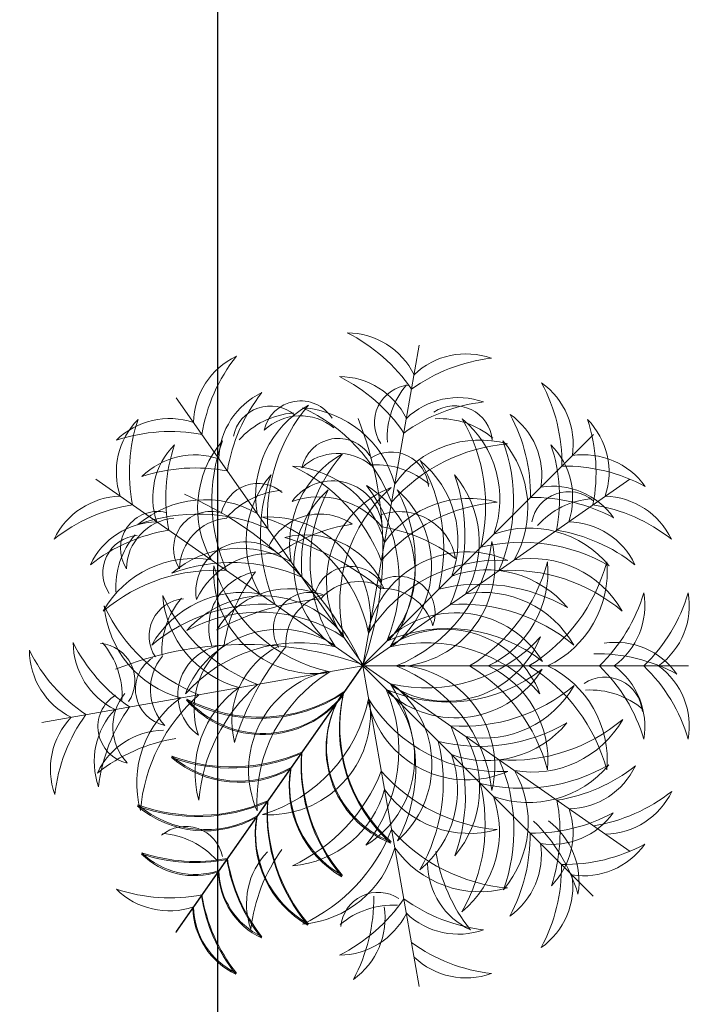
# Model space of a CAD drawing. Units: inches. Extents: x -48 to 50072, y 0 to 21068.
# Tile 18 of 75: x 289 to 316, y 309 to 347. Entities that reach past the tile are written whole.
import ezdxf

# ---------------------------------------------------------------- set-up
doc = ezdxf.new("R2010")
doc.units = ezdxf.units.IN
doc.header["$MEASUREMENT"] = 0
doc.layers.add('A-ANNO-DIMS', color=2, linetype='Continuous', lineweight=18)
doc.layers.add('L-PLNT', color=94, linetype='Continuous', lineweight=13)
doc.styles.get("Standard").update_dxf_attribs({"font": 'arial.ttf'})
doc.dimstyles.get("Standard").update_dxf_attribs({"dimtxt": 8, "dimasz": 0.18, "dimexe": 0.18, "dimexo": 0.0625, "dimgap": 0.09, "dimtad": 0, "dimtih": 1, "dimtoh": 1, "dimdec": 1, "dimzin": 0, "dimdsep": 46, "dimlunit": 4, "dimtxsty": 'Standard', "dimblk": 'ARCHTICK', "dimcen": 0.09, "dimadec": 0, "dimazin": 0, "dimtfac": 1, "dimtdec": 1, "dimtofl": 0, "dimtmove": 0, "dimatfit": 3, "dimldrblk": 'ARCHTICK', "dimfxl": 1, "dimtolj": 1, "dimtzin": 0, "dimarcsym": 0})

# ---------------------------------------------------------------- blocks, each defined once
blk = doc.blocks.new('A$C5D061C3B')
for p, q in [((3.3772, 6.6792), (3.3772, 3.3772)), ((1.4832, 6.082), (3.3772, 3.3772)), ((5.2591, 6.0863), (3.3651, 3.3814)), ((1.0302, 5.7163), (3.3651, 3.3814)), ((5.712, 5.712), (3.3772, 3.3772)), ((0.1253, 3.9506), (3.3772, 3.3772)), ((6.629, 3.9506), (3.3772, 3.3772)), ((0.6603, 1.4875), (3.3651, 3.3814)), ((1.4832, 0.6723), (3.3772, 3.3772)), ((6.0699, 1.4875), (3.3651, 3.3814)), ((3.9506, 0.1253), (3.3772, 3.3772)), ((6.082, 1.4832), (3.3772, 3.3772))]:
    blk.add_line(p, q)
for centre, radius, start, end in [((2.7629, 5.9242), 0.7621, 36.28997, 99.62433), ((2.1448, 5.0319), 1.7154, 44.07628, 73.37936), ((3.9915, 5.9242), 0.7621, 80.37567, 143.71003), ((4.6096, 5.0319), 1.7154, 106.62064, 135.92372), ((2.4194, 5.816), 0.7621, 115.37567, 178.71003), ((3.4376, 5.4395), 1.7154, 141.62064, 170.92372), ((3.9007, 5.9388), 0.7621, 125.37567, 188.71003), ((4.9688, 5.7448), 1.7154, 151.62064, 180.92372), ((3.3047, 5.4438), 1.7154, 9.07628, 38.37936), ((4.3228, 5.8202), 0.7621, 1.28997, 64.62433), ((1.9984, 5.6169), 0.7621, 125.37567, 188.71003), ((3.0665, 5.4229), 1.7154, 151.62064, 180.92372), ((2.7629, 5.4738), 0.7621, 36.28997, 99.62433), ((2.1448, 4.5814), 1.7154, 44.07628, 73.37936), ((3.9915, 5.4738), 0.7621, 80.37567, 143.71003), ((4.6096, 4.5814), 1.7154, 106.62064, 135.92372), ((3.8712, 5.8319), 0.3799, 94.742, 213.74753), ((4.4474, 5.6807), 0.826, 139.61802, 183.21064), ((4.7438, 5.6126), 0.7621, 351.28997, 54.62433), ((3.6758, 5.4187), 1.7154, 359.07628, 28.37936), ((2.6778, 5.4469), 0.7621, 115.37567, 178.71003), ((3.696, 5.0705), 1.7154, 141.62064, 170.92372), ((4.0645, 5.4512), 0.7621, 1.28997, 64.62433), ((3.0463, 5.0747), 1.7154, 9.07628, 38.37936), ((3.3438, 5.0894), 1.0556, 119.60629, 189.75109), ((4.1771, 4.8688), 1.7695, 139.96343, 183.62881), ((3.3985, 5.0936), 1.0556, 350.24891, 60.39371), ((2.5652, 4.8731), 1.7695, 356.37119, 40.03657), ((2.317, 5.2983), 0.7621, 125.37567, 188.71003), ((3.385, 5.1044), 1.7154, 151.62064, 180.92372), ((3.3573, 5.1001), 1.7154, 359.07628, 28.37936), ((4.4253, 5.2941), 0.7621, 351.28997, 54.62433), ((1.413, 5.1113), 0.7621, 71.28997, 134.62433), ((3.0349, 5.0618), 1.0556, 129.60629, 199.75109), ((3.8939, 4.9893), 1.7695, 149.96343, 193.62881), ((2.4224, 4.7989), 1.0556, 25.24891, 95.39371), ((1.8663, 4.1402), 1.7695, 31.37119, 75.03657), ((4.3319, 4.7989), 1.0556, 84.60629, 154.75109), ((4.888, 4.1402), 1.7695, 104.96343, 148.62881), ((2.8484, 4.9851), 1.7695, 346.37119, 30.03657), ((3.7074, 5.0576), 1.0556, 340.24891, 50.39371), ((1.4185, 4.0258), 1.7154, 79.07628, 108.37936), ((1.9907, 5.4623), 0.3799, 139.742, 258.74753), ((2.5051, 5.7628), 0.826, 184.61802, 228.21064), ((1.1297, 4.7481), 0.7621, 81.28997, 144.62433), ((1.6714, 4.7422), 0.7621, 71.28997, 134.62433), ((3.6883, 4.5973), 1.0556, 119.60629, 189.75109), ((4.5216, 4.3768), 1.7695, 139.96343, 183.62881), ((2.2207, 4.3811), 1.7695, 356.37119, 40.03657), ((3.054, 4.6016), 1.0556, 350.24891, 60.39371), ((5.0709, 4.7465), 0.7621, 45.37567, 108.71003), ((5.5642, 4.8068), 0.7621, 80.37567, 143.71003), ((6.1823, 3.9144), 1.7154, 106.62064, 135.92372), ((5.6126, 4.7438), 0.7621, 35.37567, 98.71003), ((1.3236, 3.68), 1.7154, 89.07628, 118.37936), ((3.4596, 4.6371), 1.0556, 129.60629, 199.75109), ((4.3186, 4.5646), 1.7695, 149.96343, 193.62881), ((3.2827, 4.6328), 1.0556, 340.24891, 50.39371), ((2.4237, 4.5604), 1.7695, 346.37119, 30.03657), ((5.4187, 3.6758), 1.7154, 61.62064, 90.92372), ((1.6769, 3.6567), 1.7154, 79.07628, 108.37936), ((5.0653, 3.661), 1.7154, 71.62064, 100.92372), ((1.4482, 4.4296), 0.7621, 81.28997, 144.62433), ((2.4224, 4.1982), 1.0556, 25.24891, 95.39371), ((1.8663, 3.5396), 1.7695, 31.37119, 75.03657), ((3.8676, 4.3207), 1.029, 121.36542, 221.57406), ((4.5556, 4.2369), 1.5567, 141.81221, 203.33354), ((4.3319, 4.1982), 1.0556, 84.60629, 154.75109), ((4.888, 3.5396), 1.7695, 104.96343, 148.62881), ((2.1867, 4.2327), 1.5567, 336.66646, 38.18779), ((2.8746, 4.3165), 1.029, 318.42594, 58.63458), ((4.0352, 4.215), 1.029, 111.36542, 211.57406), ((2.7071, 4.2192), 1.029, 328.42594, 68.63458), ((2.0441, 4.0172), 1.5567, 346.66646, 48.18779), ((4.6982, 4.0129), 1.5567, 131.81221, 193.33354), ((5.2941, 4.4253), 0.7621, 35.37567, 98.71003), ((1.6421, 3.3615), 1.7154, 89.07628, 118.37936), ((1.7796, 3.9941), 1.0556, 60.24891, 130.39371), ((4.9626, 3.9984), 1.0556, 49.60629, 119.75109), ((5.1001, 3.3573), 1.7154, 61.62064, 90.92372), ((1.7019, 3.1357), 1.7695, 66.37119, 110.03657), ((5.0404, 3.1399), 1.7695, 69.96343, 113.62881), ((2.1429, 4.5643), 1.0556, 164.60629, 234.75109), ((2.888, 4.9976), 1.7695, 184.96343, 228.62881), ((3.25, 4.4348), 1.029, 156.36542, 256.57406), ((3.8617, 4.7608), 1.5567, 176.81221, 238.33354), ((2.8927, 4.7608), 1.5567, 301.66646, 3.18779), ((3.5043, 4.4348), 1.029, 283.42594, 23.63458), ((3.8663, 4.9976), 1.7695, 311.37119, 355.03657), ((4.6115, 4.5643), 1.0556, 305.24891, 15.39371), ((1.6965, 4.1589), 0.826, 139.61802, 183.21064), ((1.6847, 3.7116), 1.0556, 70.24891, 140.39371), ((2.7344, 4.46), 1.0556, 164.60629, 234.75109), ((3.4796, 4.8933), 1.7695, 184.96343, 228.62881), ((2.3576, 3.686), 1.029, 3.42594, 103.63458), ((4.3967, 3.686), 1.029, 76.36542, 176.57406), ((3.2748, 4.8933), 1.7695, 311.37119, 355.03657), ((4.02, 4.46), 1.0556, 305.24891, 15.39371), ((5.0576, 3.7074), 1.0556, 39.60629, 109.75109), ((0.9755, 4.4244), 0.7621, 160.37567, 223.71003), ((1.9616, 4.8782), 1.7154, 186.62064, 215.92372), ((1.4191, 4.3462), 0.7621, 160.37567, 223.71003), ((2.4052, 4.8), 1.7154, 186.62064, 215.92372), ((1.1202, 4.3101), 0.3799, 94.742, 213.74753), ((1.7572, 2.8527), 1.7695, 76.37119, 120.03657), ((1.9304, 3.1403), 1.5567, 21.66646, 83.18779), ((4.8239, 3.1403), 1.5567, 96.81221, 158.33354), ((4.9851, 2.8484), 1.7695, 59.96343, 103.62881), ((4.3491, 4.8), 1.7154, 324.07628, 353.37936), ((5.3352, 4.3462), 0.7621, 316.28997, 19.62433), ((4.7927, 4.8782), 1.7154, 324.07628, 353.37936), ((5.7789, 4.4244), 0.7621, 316.28997, 19.62433), ((2.1242, 3.5021), 1.0556, 60.24891, 130.39371), ((4.6181, 3.5064), 1.0556, 49.60629, 119.75109), ((2.0464, 2.6436), 1.7695, 66.37119, 110.03657), ((4.6959, 2.6479), 1.7695, 69.96343, 113.62881), ((4.9885, 5.8124), 1.7154, 279.07628, 308.37936), ((5.3649, 4.7942), 0.7621, 271.28997, 334.62433), ((2.1094, 3.2869), 1.0556, 70.24891, 140.39371), ((2.3872, 3.7525), 0.574, 99.98654, 199.40339), ((3.5988, 3.3144), 1.651, 142.57587, 170.89417), ((4.6328, 3.2827), 1.0556, 39.60629, 109.75109), ((2.1819, 2.428), 1.7695, 76.37119, 120.03657), ((4.5604, 2.4237), 1.7695, 59.96343, 103.62881), ((2.8402, 3.7391), 0.3717, 69.22575, 210.12788), ((1.5885, 3.6663), 0.3799, 94.742, 213.74753), ((2.1647, 3.515), 0.826, 139.61802, 183.21064), ((2.3649, 3.0454), 1.029, 38.42594, 138.63458), ((3.1091, 3.5901), 0.5151, 105.43977, 183.66943), ((4.3774, 3.0496), 1.029, 41.36542, 141.57406), ((0.7621, 3.2145), 0.7621, 116.28997, 179.62433), ((2.4258, 2.8789), 1.029, 48.42594, 148.63458), ((2.3279, 2.3533), 1.5567, 56.66646, 118.18779), ((4.4143, 2.3575), 1.5567, 61.81221, 123.33354), ((4.3165, 2.8746), 1.029, 31.36542, 131.57406), ((1.5336, 2.4508), 1.7154, 124.07628, 153.37936), ((1.2058, 3.1363), 0.7621, 116.28997, 179.62433), ((1.0616, 4.4517), 0.826, 229.61802, 273.21064), ((0.9103, 3.8754), 0.3799, 184.742, 303.74753), ((5.5486, 3.1363), 0.7621, 0.37567, 63.71003), ((1.9772, 2.3726), 1.7154, 124.07628, 153.37936), ((1.8113, 2.6838), 1.0556, 105.24891, 175.39371), ((2.5096, 2.1909), 1.5567, 66.66646, 128.18779), ((4.2327, 2.1867), 1.5567, 51.81221, 113.33354), ((4.9431, 2.6838), 1.0556, 4.60629, 74.75109), ((6.0526, 3.5327), 0.3799, 146.25247, 265.258), ((4.7771, 2.3726), 1.7154, 26.62064, 55.92372), ((6.6289, 3.6839), 0.826, 176.78936, 220.38198), ((2.3633, 2.0218), 1.7695, 111.37119, 155.03657), ((2.4028, 2.5795), 1.0556, 105.24891, 175.39371), ((2.7293, 4.7024), 1.5567, 221.81221, 283.33354), ((2.5273, 4.0394), 1.029, 201.36542, 301.57406), ((4.0009, 4.7024), 1.5567, 256.66646, 318.18779), ((4.0129, 4.6982), 1.5567, 256.66646, 318.18779), ((4.2029, 4.0394), 1.029, 238.42594, 338.63458), ((4.215, 4.0352), 1.029, 238.42594, 338.63458), ((4.3515, 2.5795), 1.0556, 4.60629, 74.75109), ((4.391, 2.0218), 1.7695, 24.96343, 68.62881), ((5.9345, 2.8416), 0.7621, 35.37567, 98.71003), ((2.1851, 0.015), 3.5672, 70.47721, 111.6585), ((2.9548, 1.9175), 1.7695, 111.37119, 155.03657), ((2.0067, 3.0714), 0.5057, 93.87442, 233.97626), ((2.4891, 2.9324), 0.8252, 128.75364, 199.09705), ((2.9034, 2.8005), 0.8553, 116.44767, 194.36723), ((4.7443, 1.7792), 2.7893, 140.40074, 163.13904), ((2.7415, 3.2534), 0.3717, 114.22575, 255.12788), ((3.0371, 3.3382), 0.5151, 150.43977, 228.66943), ((3.7995, 1.9175), 1.7695, 24.96343, 68.62881), ((1.4473, 3.129), 0.3765, 122.05775, 257.85325), ((1.7505, 3.1258), 0.5286, 140.18449, 223.65396), ((2.896, 2.4268), 1.029, 83.42594, 183.63458), ((3.3592, 1.9113), 1.5567, 101.66646, 163.18779), ((3.3951, 1.9113), 1.5567, 16.81221, 78.33354), ((3.8584, 2.4268), 1.029, 356.36542, 96.57406), ((5.7406, 1.7735), 1.7154, 61.62064, 90.92372), ((4.9116, 0.1568), 3.5672, 115.47721, 156.6585), ((6.7273, 2.1893), 3.5672, 160.47721, 201.6585), ((2.4118, 2.9425), 0.574, 144.98654, 244.40339), ((3.5783, 3.4895), 1.651, 187.57587, 215.89417), ((2.1449, 3.6925), 1.0556, 209.60629, 279.75109), ((2.3655, 4.5259), 1.7695, 229.96343, 273.62881), ((2.3279, 4.401), 1.5567, 241.81221, 303.33354), ((3.6969, 2.3691), 1.029, 128.42594, 228.63458), ((4.389, 2.3322), 1.5567, 146.66646, 208.18779), ((4.6982, 2.7414), 1.5567, 166.66646, 228.18779), ((2.3412, 2.3322), 1.5567, 331.81221, 33.33354), ((2.3533, 2.3279), 1.5567, 331.81221, 33.33354), ((3.0333, 2.3691), 1.029, 311.36542, 51.57406), ((3.0454, 2.3649), 1.029, 311.36542, 51.57406), ((4.3647, 4.5259), 1.7695, 266.37119, 310.03657), ((4.3768, 4.5216), 1.7695, 266.37119, 310.03657), ((4.5853, 3.6925), 1.0556, 260.24891, 330.39371), ((4.5973, 3.6883), 1.0556, 260.24891, 330.39371), ((1.0668, 2.7485), 0.3765, 122.05775, 257.85325), ((1.3701, 2.7454), 0.5286, 140.18449, 223.65396), ((2.3649, 3.7089), 1.029, 221.36542, 321.57406), ((1.9113, 3.3592), 1.5567, 286.81221, 348.33354), ((2.4268, 2.896), 1.029, 266.36542, 6.57406), ((4.0352, 2.5394), 1.029, 148.42594, 248.63458), ((4.4348, 3.25), 1.029, 193.42594, 293.63458), ((4.7608, 3.8617), 1.5567, 211.66646, 273.18779), ((3.45, 2.6344), 0.8553, 161.44767, 239.36723), ((3.0031, 2.8444), 0.3717, 159.22575, 300.12788), ((3.1522, 3.1134), 0.5151, 195.43977, 273.66943), ((5.4738, 3.2139), 2.7893, 185.40074, 208.13904), ((1.8734, 4.1813), 1.7695, 229.96343, 273.62881), ((1.6529, 3.348), 1.0556, 209.60629, 279.75109), ((4.8568, 4.1813), 1.7695, 266.37119, 310.03657), ((4.8688, 4.1771), 1.7695, 266.37119, 310.03657), ((5.0773, 3.348), 1.0556, 260.24891, 330.39371), ((5.0894, 3.3438), 1.0556, 260.24891, 330.39371), ((4.0986, 2.0506), 1.7695, 156.37119, 200.03657), ((2.6316, 2.0506), 1.7695, 339.96343, 23.62881), ((2.6436, 2.0464), 1.7695, 339.96343, 23.62881), ((1.1216, 2.4409), 0.3799, 139.742, 258.74753), ((1.636, 2.7415), 0.826, 184.61802, 228.21064), ((3.2401, 2.1284), 1.0556, 150.24891, 220.39371), ((4.9631, 4.7486), 2.7893, 230.40074, 253.13904), ((3.4901, 2.1284), 1.0556, 319.60629, 29.75109), ((3.5021, 2.1242), 1.0556, 319.60629, 29.75109), ((1.9079, 2.3168), 0.3799, 139.742, 258.74753), ((2.4223, 2.6173), 0.826, 184.61802, 228.21064), ((2.6243, 2.1919), 0.5057, 138.87442, 278.97626), ((3.0637, 2.4347), 0.8252, 173.75364, 244.09705), ((3.9418, 2.9077), 0.8553, 206.44767, 284.36723), ((6.244, 3.9482), 1.7154, 234.07628, 263.37936), ((2.0464, 4.1107), 1.7695, 249.96343, 293.62881), ((2.1242, 3.2522), 1.0556, 229.60629, 299.75109), ((3.6066, 1.7061), 1.7695, 156.37119, 200.03657), ((4.5216, 2.3775), 1.7695, 176.37119, 220.03657), ((3.1236, 1.7061), 1.7695, 339.96343, 23.62881), ((3.1357, 1.7019), 1.7695, 339.96343, 23.62881), ((5.7902, 2.9621), 0.7621, 226.28997, 289.62433), ((1.6718, 3.7002), 1.7154, 231.62064, 260.92372), ((1.2953, 2.6821), 0.7621, 205.37567, 268.71003), ((2.7481, 1.7839), 1.0556, 150.24891, 220.39371), ((3.6883, 2.157), 1.0556, 170.24891, 240.39371), ((1.9175, 2.9548), 1.7695, 294.96343, 338.62881), ((4.8933, 3.4796), 1.7695, 221.37119, 265.03657), ((3.9821, 1.7839), 1.0556, 319.60629, 29.75109), ((3.9941, 1.7796), 1.0556, 319.60629, 29.75109), ((5.0584, 3.7002), 1.7154, 279.07628, 308.37936), ((5.0705, 3.696), 1.7154, 279.07628, 308.37936), ((5.4349, 2.6821), 0.7621, 271.28997, 334.62433), ((5.4469, 2.6778), 0.7621, 271.28997, 334.62433), ((3.4279, 3.6031), 1.651, 232.57587, 260.89417), ((2.9898, 2.3915), 0.574, 189.98654, 289.40339), ((0.9263, 2.4237), 0.7621, 205.37567, 268.71003), ((1.3028, 3.4418), 1.7154, 231.62064, 260.92372), ((2.5795, 2.4028), 1.0556, 274.60629, 344.75109), ((4.46, 2.7344), 1.0556, 215.24891, 285.39371), ((5.4274, 3.4418), 1.7154, 279.07628, 308.37936), ((5.8039, 2.4237), 0.7621, 271.28997, 334.62433), ((1.7019, 3.6187), 1.7695, 249.96343, 293.62881), ((3.0855, 1.6812), 1.7154, 169.07628, 198.37936), ((2.4047, 2.0492), 0.5286, 185.18449, 268.65396), ((4.1771, 1.8855), 1.7695, 176.37119, 220.03657), ((3.6447, 1.6812), 1.7154, 341.62064, 10.92372), ((3.6567, 1.6769), 1.7154, 341.62064, 10.92372), ((5.4395, 3.4376), 1.7154, 279.07628, 308.37936), ((5.816, 2.4194), 0.7621, 271.28997, 334.62433), ((1.7796, 2.7602), 1.0556, 229.60629, 299.75109), ((2, 1.6757), 0.7621, 161.28997, 224.62433), ((2.188, 1.837), 0.3765, 167.05775, 302.85325), ((3.8099, 2.4933), 0.8252, 218.75364, 289.09705), ((3.6709, 2.011), 0.5057, 183.87442, 323.97626), ((5.3845, 1.5838), 0.3799, 101.25247, 220.258), ((5.8989, 1.2832), 0.826, 131.78936, 175.38198), ((4.7302, 1.6757), 0.7621, 315.37567, 18.71003), ((4.7422, 1.6714), 0.7621, 315.37567, 18.71003), ((3.3438, 1.665), 1.0556, 170.24891, 240.39371), ((2.7165, 1.4228), 1.7154, 169.07628, 198.37936), ((2.0218, 2.3633), 1.7695, 294.96343, 338.62881), ((4.9976, 2.888), 1.7695, 221.37119, 265.03657), ((4.0137, 1.4228), 1.7154, 341.62064, 10.92372), ((1.631, 1.4173), 0.7621, 161.28997, 224.62433), ((5.0992, 1.4173), 0.7621, 315.37567, 18.71003), ((3.2272, 2.169), 0.826, 229.61802, 273.21064), ((3.076, 1.5927), 0.3799, 184.742, 303.74753), ((2.6838, 1.8113), 1.0556, 274.60629, 344.75109), ((4.5643, 2.1429), 1.0556, 215.24891, 285.39371), ((1.6714, 2.0121), 0.7621, 225.37567, 288.71003), ((1.6769, 3.0976), 1.7154, 251.62064, 280.92372), ((2.4047, 1.5112), 0.5286, 185.18449, 268.65396), ((3.696, 1.6838), 1.7154, 189.07628, 218.37936), ((5.8081, 1.7538), 1.7154, 189.07628, 218.37936), ((2.188, 1.299), 0.3765, 167.05775, 302.85325), ((3.6165, 1.7548), 0.5286, 230.18449, 313.65396), ((3.6133, 1.4515), 0.3765, 212.05775, 347.85325), ((4.79, 1.3774), 0.7621, 181.28997, 244.62433), ((2.6778, 1.3074), 0.7621, 181.28997, 244.62433), ((1.4185, 2.7286), 1.7154, 251.62064, 280.92372), ((1.413, 1.6431), 0.7621, 225.37567, 288.71003), ((3.4376, 1.3148), 1.7154, 189.07628, 218.37936), ((2.5834, 1.7007), 0.826, 229.61802, 273.21064), ((2.4322, 1.1245), 0.3799, 184.742, 303.74753), ((2.3726, 1.9772), 1.7154, 296.62064, 325.92372), ((3.5285, 0.6896), 0.3799, 56.25247, 175.258), ((4.8, 2.4052), 1.7154, 234.07628, 263.37936), ((2.4194, 0.9384), 0.7621, 181.28997, 244.62433), ((3.6797, 0.1134), 0.826, 86.78936, 130.38198), ((3.9969, 1.3743), 0.5286, 230.18449, 313.65396), ((3.9938, 1.0711), 0.3765, 212.05775, 347.85325), ((3.1363, 1.2058), 0.7621, 270.37567, 333.71003), ((4.3462, 1.4191), 0.7621, 226.28997, 289.62433), ((2.4508, 1.5336), 1.7154, 296.62064, 325.92372), ((4.8782, 1.9616), 1.7154, 234.07628, 263.37936), ((3.2145, 0.7621), 0.7621, 270.37567, 333.71003), ((4.4244, 0.9755), 0.7621, 226.28997, 289.62433)]:
    blk.add_arc(centre, radius, start, end)
blk = doc.blocks.new('_ArchTick')
at = {"color": 0, "linetype": 'ByBlock', "const_width": 0.15}
blk.add_lwpolyline([(-0.5, -0.5), (0.5, 0.5)], dxfattribs=at)
blk = doc.blocks.new('*D117')
at = {"layer": 'A-ANNO-DIMS', "color": 0, "lineweight": -2, "transparency": 16777216}
for p, q in [((216.017, 488.712), (216.017, 165.945)), ((297.017, 488.712), (297.017, 165.945)), ((216.017, 166.125), (251.464, 166.125)), ((297.017, 166.125), (261.57, 166.125))]:
    blk.add_line(p, q, dxfattribs=at)
at = {"layer": 'Defpoints', "color": 0, "transparency": 16777216}
for p in [(216.017, 488.775), (297.017, 488.775), (297.017, 166.125)]:
    blk.add_point(p, dxfattribs=at)
at = {"layer": 'A-ANNO-DIMS', "color": 0, "lineweight": -2, "transparency": 16777216, "xscale": 0.18, "yscale": 0.18, "zscale": 0.18, "rotation": 180}
blk.add_blockref('_ArchTick', (216.017, 166.125), dxfattribs=at)
at = {"layer": 'A-ANNO-DIMS', "color": 0, "lineweight": -2, "transparency": 16777216, "xscale": 0.18, "yscale": 0.18, "zscale": 0.18}
blk.add_blockref('_ArchTick', (297.017, 166.125), dxfattribs=at)
at = {"layer": 'A-ANNO-DIMS', "color": 0, "transparency": 16777216, "insert": (256.517, 166.125), "char_height": 8, "attachment_point": 5}
blk.add_mtext('\\A1;81', dxfattribs=at)
blk = doc.blocks.new('*D118')
at = {"layer": 'A-ANNO-DIMS', "color": 0, "lineweight": -2, "transparency": 16777216}
for p, q in [((297.017, 488.712), (297.017, 165.945)), ((463.517, 488.712), (463.517, 165.945)), ((297.017, 166.125), (367.026, 166.125)), ((463.517, 166.125), (393.509, 166.125))]:
    blk.add_line(p, q, dxfattribs=at)
at = {"layer": 'Defpoints', "color": 0, "transparency": 16777216}
for p in [(297.017, 488.775), (463.517, 488.775), (463.517, 166.125)]:
    blk.add_point(p, dxfattribs=at)
at = {"layer": 'A-ANNO-DIMS', "color": 0, "lineweight": -2, "transparency": 16777216, "xscale": 0.18, "yscale": 0.18, "zscale": 0.18, "rotation": 180}
blk.add_blockref('_ArchTick', (297.017, 166.125), dxfattribs=at)
at = {"layer": 'A-ANNO-DIMS', "color": 0, "lineweight": -2, "transparency": 16777216, "xscale": 0.18, "yscale": 0.18, "zscale": 0.18}
blk.add_blockref('_ArchTick', (463.517, 166.125), dxfattribs=at)
at = {"layer": 'A-ANNO-DIMS', "color": 0, "transparency": 16777216, "insert": (380.267, 166.125), "char_height": 8, "attachment_point": 5}
blk.add_mtext('\\A1;166.5', dxfattribs=at)

msp = doc.modelspace()

# ---------------------------------------------------------------- block references
at = {"layer": 'L-PLNT', "xscale": 3.862191520948588, "yscale": 3.862191520948588, "zscale": 3.862191520948588, "rotation": 270}
msp.add_blockref('A$C5D061C3B', (289.656, 335.046), dxfattribs=at)

# ---------------------------------------------------------------- dimensions: what is measured, and where the dimension line sits
at = {"layer": 'A-ANNO-DIMS'}
for base, p1, p2, override, picture, middle in [((297.017, 166.125), (216.017, 488.775), (297.017, 488.775), {"dimdec": 0, "dimlfac": 1, "dimrnd": 0, "dimzin": 0, "dimdsep": 46, "dimlunit": 2}, '*D117', (256.517, 166.125)), ((463.517, 166.125), (297.017, 488.775), (463.517, 488.775), {"dimdec": 1, "dimlfac": 1, "dimrnd": 0, "dimzin": 0, "dimdsep": 46, "dimlunit": 2}, '*D118', (380.267, 166.125))]:
    dim = msp.add_linear_dim(base=base, p1=p1, p2=p2, dimstyle='Standard', override=override, dxfattribs=at)
    dim.commit()
    dim.dimension.update_dxf_attribs({"geometry": picture, "text_midpoint": middle})

doc.saveas('drawing.dxf')
